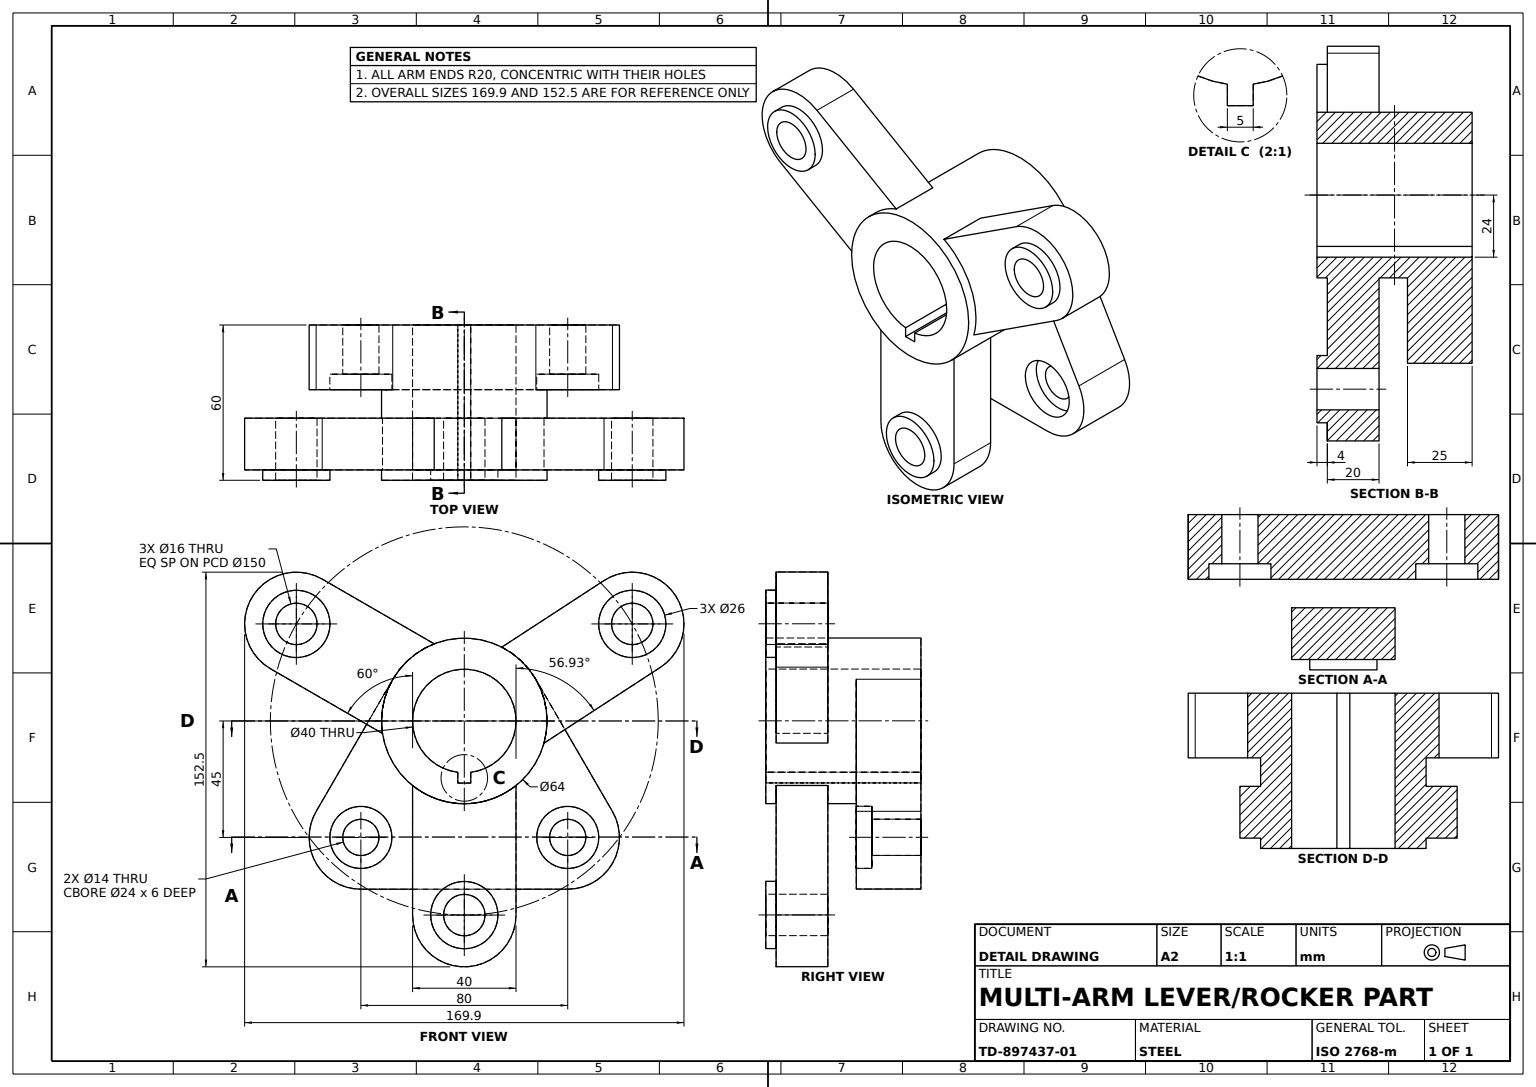
SolidWorks part; units mm, degrees
material "Plain Carbon Steel"
ref_plane "Front Plane" through (0, 0, 0) normal (0, 0, 1) x (1, 0, 0)
ref_plane "Top Plane" through (0, 0, 0) normal (0, 1, 0) x (1, 0, 0)
ref_plane "Right Plane" through (0, 0, 0) normal (1, 0, 0) x (0, 0, -1)
sketch "Lower Arms Profile" plane through (0, 0, 0) normal (0, 0, 1) x (1, 0, 0)
  line L0 (0, 0) -> (0, -45)
  line L1 (0, -45) -> (-40, -45)
  line L2 (0, -45) -> (40, -45)
  line L3 (-57.2966, -34.9586) -> (-27.6745, 16.0662)
  line L4 (27.6745, 16.0662) -> (57.2966, -34.9586)
  line L5 (-40, -65) -> (40, -65)
  arc A0 (27.6745, 16.0662) -> (-27.6745, 16.0662) centre (0, 0) ccw
  arc A1 (-57.2966, -34.9586) -> (-40, -65) centre (-40, -45) ccw
  arc A2 (40, -65) -> (57.2966, -34.9586) centre (40, -45) ccw
  dimension "D1" = 32
  dimension "D5" = 20
  dimension "D6" = 20
  dimension "D2" = 45
  dimension "D3" = 40
  dimension "D4" = 40
extrude "Lower Arms 25mm" add sketch "Lower Arms Profile" along normal blind 25
sketch "Hub Boss Sketch Ø32" plane through (0, 0, 25) normal (0, 0, 1) x (1, 0, 0)
  circle A0 centre (0, 0) radius 32
  dimension "D1" = 32
extrude "Hub Boss Ø32" add sketch "Hub Boss Sketch Ø32" along normal blind 31
sketch "Upper Arms Profile" plane through (0, 0, 56) normal (0, 0, 1) x (1, 0, 0)
  line L0 (-20, -75) -> (-20, -24.98)
  line L1 (20, -75) -> (20, -24.98)
  line L2 (0, 0) -> (0, 95.4956) construction
  line L3 (0, 0) -> (64.9519, 37.5) construction
  line L4 (0, 0) -> (-64.9519, 37.5) construction
  line L6 (-74.9519, 20.1795) -> (-31.6333, -4.8305)
  line L8 (-54.9519, 54.8205) -> (-11.6333, 29.8105)
  line L9 (54.0396, 54.2607) -> (14.5072, 28.5226)
  line L10 (75.8642, 20.7393) -> (30.8276, -8.5823)
  circle A0 centre (0, 0) radius 75 construction
  arc A1 (-19.8214, -72.3333) -> (19.8214, -72.3333) centre (0, -75) ccw
  arc A2 (-20, -24.98) -> (20, -24.98) centre (0, 0) ccw
  arc A3 (-54.9519, 54.8205) -> (-74.9519, 20.1795) centre (-64.9519, 37.5) ccw
  arc A4 (75.8642, 20.7393) -> (54.0396, 54.2607) centre (64.9519, 37.5) ccw
  circle A5 centre (0, 0) radius 32 construction
  arc A6 (-20, -24.98) -> (20, -24.98) centre (0, 0) ccw
  arc A7 (-11.6333, 29.8105) -> (-31.6333, -4.8305) centre (0, 0) ccw
  arc A8 (30.8276, -8.5823) -> (14.5072, 28.5226) centre (0, 0) ccw
  dimension "D1" = 75
  dimension "D2" = 20
  dimension "D3" = 43.3186
  dimension "D4" = 60
  dimension "D6" = 20
  dimension "D7" = 20
  dimension "D8" = 20
  dimension "D10" = 20
  dimension "D12" = 39.5324
  dimension "D5" = 60
  dimension "D9" = 40
  dimension "D11" = 25.01
extrude "Upper Arms 20mm" add sketch "Upper Arms Profile" against normal blind 20
sketch "Hub Collar Sketch Ø32" plane through (0, 0, 56) normal (0, 0, 1) x (1, 0, 0)
  circle A0 centre (0, 0) radius 32
  dimension "D1" = 32
extrude "Hub Collar Ø32x4" add sketch "Hub Collar Sketch Ø32" along normal blind 4
sketch "Keyed Bore Sketch" plane through (0, 0, 60) normal (0, 0, 1) x (1, 0, 0)
  line L0 (-2.5, -24) -> (2.5, -24)
  line L2 (2.5, -24) -> (2.5, -19.8431)
  line L4 (-2.5, -24) -> (-2.5, -19.8431)
  arc A0 (2.5, -19.8431) -> (-2.5, -19.8431) centre (0, 0) ccw
  dimension "D1" = 20
  dimension "D2" = 5
  dimension "D3" = 4.1569
  dimension "D4" = 24
extrude "Keyed Hub Bore" cut sketch "Keyed Bore Sketch" against normal blind 70
sketch "Upper Arm Pads Sketch 3xØ13" plane through (0, 0, 56) normal (0, 0, 1) x (1, 0, 0)
  circle A0 centre (-64.9519, 37.5) radius 13
  circle A1 centre (64.9519, 37.5) radius 13
  circle A2 centre (0, -75) radius 13
  dimension "D1" = 13
  dimension "D2" = 13
  dimension "D3" = 13
extrude "Upper Arm Pads 3xØ13" add sketch "Upper Arm Pads Sketch 3xØ13" along normal blind 4
sketch "Upper Arm Holes Sketch 3xØ8" plane through (0, 0, 60) normal (0, 0, 1) x (1, 0, 0)
  circle A0 centre (-64.9519, 37.5) radius 8
  circle A1 centre (64.9519, 37.5) radius 8
  circle A2 centre (0, -75) radius 8
  dimension "D1" = 8
  dimension "D2" = 8
  dimension "D3" = 8
extrude "Upper Arm Holes 3xØ8" cut sketch "Upper Arm Holes Sketch 3xØ8" against normal blind 30
sketch "Lower Arm Counterbores Sketch 2xØ12" plane through (0, 0, 25) normal (0, 0, 1) x (1, 0, 0)
  circle A0 centre (-40, -45) radius 12
  circle A1 centre (40, -45) radius 12
  dimension "D1" = 12
  dimension "D2" = 12
extrude "Lower Arm Counterbores 2xØ12" cut sketch "Lower Arm Counterbores Sketch 2xØ12" against normal blind 6
sketch "Lower Arm Holes Sketch 2xØ7" plane through (0, 0, 19) normal (0, 0, 1) x (1, 0, 0)
  circle A0 centre (-40, -45) radius 7
  circle A1 centre (40, -45) radius 7
  dimension "D1" = 7
  dimension "D2" = 7
extrude "Lower Arm Holes 2xØ7" cut sketch "Lower Arm Holes Sketch 2xØ7" against normal blind 20
